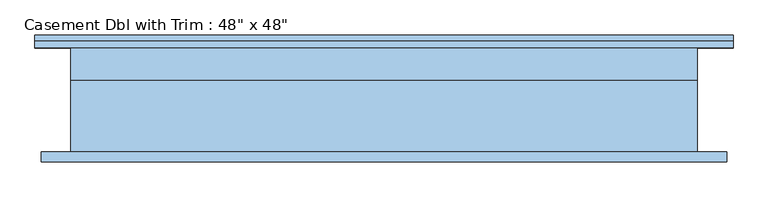
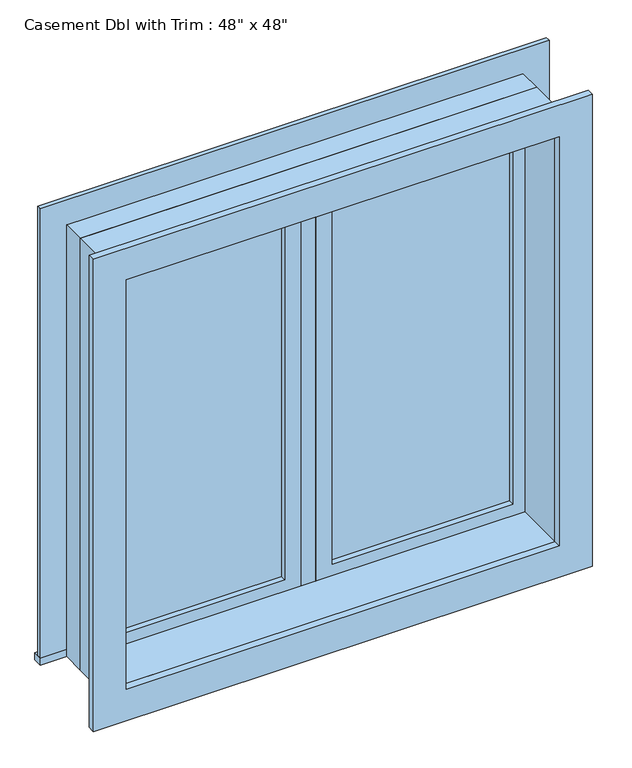
"""IFC4 building model written with IfcOpenShell, lengths in millimetres: window geometry."""

from ifc_helpers import new_model, si_unit, frame, origin, place, context, project, spatial, polyline, outline, extrude, source, transform, mapped, element, save


def window_0862ab64(model_context):
    return source(origin(), model_context, "Body", "SweptSolid", [
        extrude(outline(polyline([(63.5, 85.725), (546.1, 85.725), (546.1, 73.025), (63.5, 73.025), (63.5, 85.725)])), frame((0.0, 0.0, 977.9), z_axis=(0.0, 0.0, 1.0), x_axis=(1.0, 0.0, 0.0)), (0.0, 0.0, 1.0), 1092.2),
        extrude(outline(polyline([(2114.55, 19.05), (933.45, 19.05), (933.45, 590.55), (2114.55, 590.55), (2114.55, 19.05)]), holes=[polyline([(2070.1, 63.5), (2070.1, 546.1), (977.9, 546.1), (977.9, 63.5), (2070.1, 63.5)])]), frame((0.0, 57.15, 0.0), z_axis=(0.0, 1.0, 0.0), x_axis=(0.0, 0.0, 1.0)), (0.0, 0.0, 1.0), 44.45),
        extrude(outline(polyline([(19.05, 57.15), (-19.05, 57.15), (-19.05, 120.65), (19.05, 120.65), (19.05, 57.15)])), frame((0.0, 0.0, 933.45), z_axis=(0.0, 0.0, 1.0), x_axis=(1.0, 0.0, 0.0)), (0.0, 0.0, 1.0), 1181.1),
        extrude(outline(polyline([(-679.45, 146.05), (679.45, 146.05), (679.45, 120.65), (-679.45, 120.65), (-679.45, 146.05)])), frame((0.0, 0.0, 914.4), z_axis=(0.0, 0.0, 1.0), x_axis=(1.0, 0.0, 0.0)), (0.0, 0.0, 1.0), 19.05),
        extrude(outline(polyline([(2114.55, -590.55), (2114.55, 590.55), (933.45, 590.55), (933.45, 679.45), (2203.45, 679.45), (2203.45, -679.45), (933.45, -679.45), (933.45, -590.55), (2114.55, -590.55)])), frame((0.0, 120.65, 0.0), z_axis=(0.0, 1.0, 0.0), x_axis=(0.0, 0.0, 1.0)), (0.0, 0.0, 1.0), 12.7),
        extrude(outline(polyline([(2190.75, 666.75), (2190.75, -666.75), (857.25, -666.75), (857.25, 666.75), (2190.75, 666.75)]), holes=[polyline([(2101.85, 577.85), (946.15, 577.85), (946.15, -577.85), (2101.85, -577.85), (2101.85, 577.85)])]), frame((0.0, -101.6, 0.0), z_axis=(0.0, 1.0, 0.0), x_axis=(0.0, 0.0, 1.0)), (0.0, 0.0, 1.0), 19.05),
        extrude(outline(polyline([(-63.5, 73.025), (-546.1, 73.025), (-546.1, 85.725), (-63.5, 85.725), (-63.5, 73.025)])), frame((0.0, 0.0, 977.9), z_axis=(0.0, 0.0, 1.0), x_axis=(1.0, 0.0, 0.0)), (0.0, 0.0, 1.0), 1092.2),
        extrude(outline(polyline([(2114.55, -590.55), (933.45, -590.55), (933.45, -19.05), (2114.55, -19.05), (2114.55, -590.55)]), holes=[polyline([(2070.1, -546.1), (2070.1, -63.5), (977.9, -63.5), (977.9, -546.1), (2070.1, -546.1)])]), frame((0.0, 57.15, 0.0), z_axis=(0.0, 1.0, 0.0), x_axis=(0.0, 0.0, 1.0)), (0.0, 0.0, 1.0), 44.45),
        extrude(outline(polyline([(2133.6, -609.6), (914.4, -609.6), (914.4, 609.6), (2133.6, 609.6), (2133.6, -609.6)]), holes=[polyline([(2101.85, -577.85), (2101.85, 577.85), (946.15, 577.85), (946.15, -577.85), (2101.85, -577.85)])]), frame((0.0, -82.55, 0.0), z_axis=(0.0, 1.0, 0.0), x_axis=(0.0, 0.0, 1.0)), (0.0, 0.0, 1.0), 139.7),
        extrude(outline(polyline([(2133.6, 609.6), (2133.6, -609.6), (914.4, -609.6), (914.4, 609.6), (2133.6, 609.6)]), holes=[polyline([(2114.55, 590.55), (933.45, 590.55), (933.45, -590.55), (2114.55, -590.55), (2114.55, 590.55)])]), frame((0.0, 57.15, 0.0), z_axis=(0.0, 1.0, 0.0), x_axis=(0.0, 0.0, 1.0)), (0.0, 0.0, 1.0), 63.5),
    ])


if __name__ == "__main__":
    model = new_model("IFC4")
    model_context = context("Model", 3, world=origin())
    ifc_project = project(units=[si_unit("LENGTHUNIT", "METRE", prefix="MILLI")], contexts=[model_context])
    site = spatial("IfcSite", under=ifc_project)
    building = spatial("IfcBuilding", under=site)
    placement = place(None, origin())
    window_shape = window_0862ab64(model_context)
    element("IfcWindow", 1, ObjectType="Casement Dbl with Trim : 48\" x 48\"", at=placement, inside=building, context=model_context, shape_type="MappedRepresentation", body=[
        mapped(window_shape, transform((0.0, 0.0, 0.0), x_axis=(1.0, 0.0, 0.0), y_axis=(0.0, 1.0, 0.0), z_axis=(0.0, 0.0, 1.0))),
    ])
    save(model, "model.ifc")

# Revit data of these elements
# Type "Casement Dbl with Trim : 48\" x 48\""
#   Type Mark = "10"
#   Construction Type Id = "GSP4R"
#   Assembly Code = "B2020100"
#   Analytic Construction = "1/8 in Pilkington single glazing"
#   Visual Light Transmittance = 0.9
#   Solar Heat Gain Coefficient = 0.78
#   Heat Transfer Coefficient (U) = 0.6496 BTU/(h·ft²·°F)
#   Height = 4' - 0"
#   Default Sill Height = 3' - 0"
#   Trim Projection - Ext. = 0' - 0 1/2"
#   Trim Projection - Int. = 0' - 0 3/4"
#   Trim Width - Exterior = 0' - 3 1/2"
#   Trim Width - Interior = 0' - 3 1/2"
#   Width = 4' - 0"
#   Window Inset = 0' - 0 3/4"
#   Define Thermal Properties by = 1
#   Glass Pane Material = Glass
#   Sash Material = Sash
#   Trim Exterior Material = Trim
#   Trim Interior Material = Trim
#   Wall Closure = (empty or 0)
# Element 1 (IfcWindow, "Casement Dbl with Trim : 48\" x 48\"")
#   Materials on its faces: "Sash", "Trim", "Glass"
# Materials
#   "Glass": class "Glass", colour RGB 0 128 192, transparency 0.75, Description = "Soda Lime Glass", Cost = 0
#   "Sash": class "Wood", colour RGB 224 178 126, transparency 0
#   "Trim": class "Wood", colour RGB 224 178 126, transparency 0
